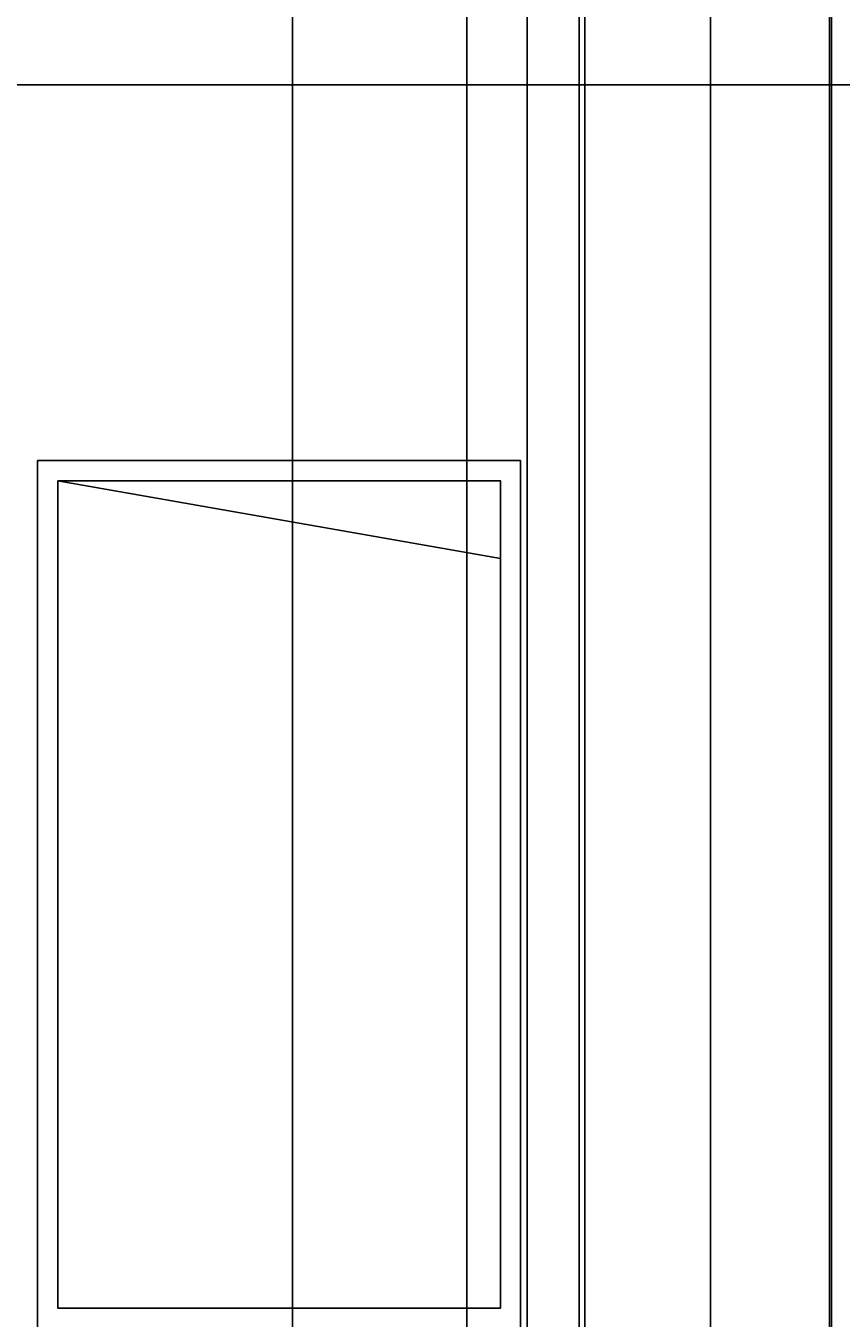
# Model space of a CAD drawing. Units: inches. Extents: x 69 to 650, y -16 to 573.
# Tile 5 of 26: x 264 to 345, y 89 to 218. Entities that reach past the tile are written whole.
import ezdxf

# ---------------------------------------------------------------- set-up
doc = ezdxf.new("R2010")
doc.units = ezdxf.units.IN
doc.header["$MEASUREMENT"] = 0
doc.layers.add('A-ANNO-DIMS', color=2, linetype='Continuous', lineweight=18)
doc.layers.add('A-DOOR', color=3, linetype='Continuous', lineweight=25)
doc.styles.get("Standard").update_dxf_attribs({"font": 'arial.ttf'})
doc.dimstyles.get("Standard").update_dxf_attribs({"dimtxt": 0.8125, "dimasz": 0.18, "dimexe": 0.18, "dimexo": 0.0625, "dimgap": 0.09, "dimtad": 0, "dimtih": 1, "dimtoh": 1, "dimdec": 4, "dimzin": 0, "dimdsep": 46, "dimlunit": 4, "dimtxsty": 'Standard', "dimcen": 0.09, "dimadec": 0, "dimazin": 0, "dimtfac": 1, "dimtdec": 4, "dimtofl": 0, "dimtmove": 0, "dimatfit": 3, "dimfxl": 1, "dimtolj": 1, "dimtzin": 0, "dimarcsym": 0})

# ---------------------------------------------------------------- blocks, each defined once
blk = doc.blocks.new('*D19')
at = {"layer": 'A-ANNO-DIMS', "color": 0, "lineweight": -2, "transparency": 16777216}
for p, q in [((99.56, 471.72), (99.56, 572.74)), ((99.74, 572.56), (358.57, 572.56)), ((619.38, 572.56), (360.54, 572.56)), ((619.56, 87.99), (619.56, 572.74))]:
    blk.add_line(p, q, dxfattribs=at)
at = {"layer": 'A-ANNO-DIMS', "color": 0, "transparency": 16777216}
for points in [[(99.74, 572.59), (99.74, 572.53), (99.56, 572.56)], [(619.38, 572.59), (619.38, 572.53), (619.56, 572.56)]]:
    blk.add_solid(points, dxfattribs=at)
at = {"layer": 'Defpoints', "color": 0, "transparency": 16777216}
for p in [(619.56, 572.56), (99.56, 471.66), (619.56, 87.93)]:
    blk.add_point(p, dxfattribs=at)
at = {"layer": 'A-ANNO-DIMS', "color": 0, "transparency": 16777216, "insert": (359.56, 572.56), "char_height": 0.812, "attachment_point": 5}
blk.add_mtext('\\A1;520', dxfattribs=at)
blk = doc.blocks.new('*D24')
at = {"layer": 'A-ANNO-DIMS', "color": 0, "lineweight": -2, "transparency": 16777216}
for p, q in [((441.88, 211.65), (70.98, 211.65)), ((71.16, 211.47), (71.16, 207.04)), ((71.16, 201.6), (71.16, 206.03)), ((173.51, 201.42), (70.98, 201.42))]:
    blk.add_line(p, q, dxfattribs=at)
at = {"layer": 'A-ANNO-DIMS', "color": 0, "transparency": 16777216}
for points in [[(71.13, 211.47), (71.19, 211.47), (71.16, 211.65)], [(71.13, 201.6), (71.19, 201.6), (71.16, 201.42)]]:
    blk.add_solid(points, dxfattribs=at)
at = {"layer": 'Defpoints', "color": 0, "transparency": 16777216}
for p in [(71.16, 211.65), (441.94, 211.65), (173.58, 201.42)]:
    blk.add_point(p, dxfattribs=at)
at = {"layer": 'A-ANNO-DIMS', "color": 0, "transparency": 16777216, "insert": (71.16, 206.54), "char_height": 0.812, "attachment_point": 5}
blk.add_mtext('\\A1;10.229', dxfattribs=at)
blk = doc.blocks.new('*D25')
at = {"layer": 'A-ANNO-DIMS', "color": 0, "lineweight": -2, "transparency": 16777216}
for p, q in [((99.49, 243.93), (70.98, 243.93)), ((71.16, 243.75), (71.16, 228.3)), ((71.16, 211.83), (71.16, 227.29)), ((441.88, 211.65), (70.98, 211.65))]:
    blk.add_line(p, q, dxfattribs=at)
at = {"layer": 'A-ANNO-DIMS', "color": 0, "transparency": 16777216}
for points in [[(71.13, 243.75), (71.19, 243.75), (71.16, 243.93)], [(71.13, 211.83), (71.19, 211.83), (71.16, 211.65)]]:
    blk.add_solid(points, dxfattribs=at)
at = {"layer": 'Defpoints', "color": 0, "transparency": 16777216}
for p in [(71.16, 243.93), (99.56, 243.93), (441.94, 211.65)]:
    blk.add_point(p, dxfattribs=at)
at = {"layer": 'A-ANNO-DIMS', "color": 0, "transparency": 16777216, "insert": (71.16, 227.79), "char_height": 0.812, "attachment_point": 5}
blk.add_mtext('\\A1;32.28', dxfattribs=at)
blk = doc.blocks.new('*D30')
at = {"layer": 'A-ANNO-DIMS', "color": 0, "lineweight": -2, "transparency": 16777216}
for p, q in [((352.94, 174.2), (352.94, 35.35)), ((313.14, 87.92), (313.14, 35.35)), ((313.32, 35.53), (331.9, 35.53)), ((352.76, 35.53), (334.19, 35.53))]:
    blk.add_line(p, q, dxfattribs=at)
at = {"layer": 'A-ANNO-DIMS', "color": 0, "transparency": 16777216}
for points in [[(313.32, 35.56), (313.32, 35.5), (313.14, 35.53)], [(352.76, 35.56), (352.76, 35.5), (352.94, 35.53)]]:
    blk.add_solid(points, dxfattribs=at)
at = {"layer": 'Defpoints', "color": 0, "transparency": 16777216}
for p in [(352.94, 174.27), (313.14, 87.99), (352.94, 35.53)]:
    blk.add_point(p, dxfattribs=at)
at = {"layer": 'A-ANNO-DIMS', "color": 0, "transparency": 16777216, "insert": (333.04, 35.53), "char_height": 0.812, "attachment_point": 5}
blk.add_mtext('\\A1;39.8', dxfattribs=at)
blk = doc.blocks.new('*D37')
at = {"layer": 'A-ANNO-DIMS', "color": 0, "lineweight": -2, "transparency": 16777216}
for p, q in [((307.8, 384.84), (307.8, 35.35)), ((290.45, 372.93), (290.45, 35.35)), ((290.63, 35.53), (297.7, 35.53)), ((307.62, 35.53), (300.55, 35.53))]:
    blk.add_line(p, q, dxfattribs=at)
at = {"layer": 'A-ANNO-DIMS', "color": 0, "transparency": 16777216}
for points in [[(290.63, 35.56), (290.63, 35.5), (290.45, 35.53)], [(307.62, 35.56), (307.62, 35.5), (307.8, 35.53)]]:
    blk.add_solid(points, dxfattribs=at)
at = {"layer": 'Defpoints', "color": 0, "transparency": 16777216}
for p in [(307.8, 384.9), (290.45, 372.99), (307.8, 35.53)]:
    blk.add_point(p, dxfattribs=at)
at = {"layer": 'A-ANNO-DIMS', "color": 0, "transparency": 16777216, "insert": (299.12, 35.53), "char_height": 0.812, "attachment_point": 5}
blk.add_mtext('\\A1;17.35', dxfattribs=at)
blk = doc.blocks.new('*D38')
at = {"layer": 'A-ANNO-DIMS', "color": 0, "lineweight": -2, "transparency": 16777216}
for p, q in [((307.8, 384.84), (307.8, 35.35)), ((390.43, 384.84), (390.43, 35.35)), ((307.98, 35.53), (347.65, 35.53)), ((390.25, 35.53), (350.57, 35.53))]:
    blk.add_line(p, q, dxfattribs=at)
at = {"layer": 'A-ANNO-DIMS', "color": 0, "transparency": 16777216}
for points in [[(307.98, 35.56), (307.98, 35.5), (307.8, 35.53)], [(390.25, 35.56), (390.25, 35.5), (390.43, 35.53)]]:
    blk.add_solid(points, dxfattribs=at)
at = {"layer": 'Defpoints', "color": 0, "transparency": 16777216}
for p in [(307.8, 384.9), (390.43, 384.9), (390.43, 35.53)]:
    blk.add_point(p, dxfattribs=at)
at = {"layer": 'A-ANNO-DIMS', "color": 0, "transparency": 16777216, "insert": (349.11, 35.53), "char_height": 0.812, "attachment_point": 5}
blk.add_mtext('\\A1;82.63', dxfattribs=at)
blk = doc.blocks.new('*D64')
at = {"layer": 'A-ANNO-DIMS', "color": 0, "lineweight": -2, "transparency": 16777216}
for p, q in [((319.55, 393.8), (319.55, 35.35)), ((344.08, 393.8), (344.08, 35.35)), ((319.73, 35.53), (330.35, 35.53)), ((343.9, 35.53), (333.28, 35.53))]:
    blk.add_line(p, q, dxfattribs=at)
at = {"layer": 'A-ANNO-DIMS', "color": 0, "transparency": 16777216}
for points in [[(319.73, 35.56), (319.73, 35.5), (319.55, 35.53)], [(343.9, 35.56), (343.9, 35.5), (344.08, 35.53)]]:
    blk.add_solid(points, dxfattribs=at)
at = {"layer": 'Defpoints', "color": 0, "transparency": 16777216}
for p in [(319.55, 393.86), (344.08, 393.86), (344.08, 35.53)]:
    blk.add_point(p, dxfattribs=at)
at = {"layer": 'A-ANNO-DIMS', "color": 0, "transparency": 16777216, "insert": (331.82, 35.53), "char_height": 0.812, "attachment_point": 5}
blk.add_mtext('\\A1;24.53', dxfattribs=at)
blk = doc.blocks.new('*D65')
at = {"layer": 'A-ANNO-DIMS', "color": 0, "lineweight": -2, "transparency": 16777216}
for p, q in [((344.08, 393.8), (344.08, 35.35)), ((368.88, 393.8), (368.88, 35.35)), ((344.26, 35.53), (355.33, 35.53)), ((368.7, 35.53), (357.63, 35.53))]:
    blk.add_line(p, q, dxfattribs=at)
at = {"layer": 'A-ANNO-DIMS', "color": 0, "transparency": 16777216}
for points in [[(344.26, 35.56), (344.26, 35.5), (344.08, 35.53)], [(368.7, 35.56), (368.7, 35.5), (368.88, 35.53)]]:
    blk.add_solid(points, dxfattribs=at)
at = {"layer": 'Defpoints', "color": 0, "transparency": 16777216}
for p in [(344.08, 393.86), (368.88, 393.86), (368.88, 35.53)]:
    blk.add_point(p, dxfattribs=at)
at = {"layer": 'A-ANNO-DIMS', "color": 0, "transparency": 16777216, "insert": (356.48, 35.53), "char_height": 0.812, "attachment_point": 5}
blk.add_mtext('\\A1;24.8', dxfattribs=at)
blk = doc.blocks.new('*D66')
at = {"layer": 'A-ANNO-DIMS', "color": 0, "lineweight": -2, "transparency": 16777216}
for p, q in [((313.81, 263.46), (313.81, 35.35)), ((318.98, 263.46), (318.98, 35.35)), ((313.99, 35.53), (314.93, 35.53)), ((318.8, 35.53), (317.85, 35.53))]:
    blk.add_line(p, q, dxfattribs=at)
at = {"layer": 'A-ANNO-DIMS', "color": 0, "transparency": 16777216}
for points in [[(313.99, 35.56), (313.99, 35.5), (313.81, 35.53)], [(318.8, 35.56), (318.8, 35.5), (318.98, 35.53)]]:
    blk.add_solid(points, dxfattribs=at)
at = {"layer": 'Defpoints', "color": 0, "transparency": 16777216}
for p in [(313.81, 263.53), (318.98, 263.53), (318.98, 35.53)]:
    blk.add_point(p, dxfattribs=at)
at = {"layer": 'A-ANNO-DIMS', "color": 0, "transparency": 16777216, "insert": (316.39, 35.53), "char_height": 0.812, "attachment_point": 5}
blk.add_mtext('\\A1;5.174', dxfattribs=at)
blk = doc.blocks.new('*D67')
at = {"layer": 'A-ANNO-DIMS', "color": 0, "lineweight": -2, "transparency": 16777216}
for p, q in [((318.98, 263.46), (318.98, 35.35)), ((332.05, 263.46), (332.05, 35.35)), ((319.16, 35.53), (324.09, 35.53)), ((331.87, 35.53), (326.94, 35.53))]:
    blk.add_line(p, q, dxfattribs=at)
at = {"layer": 'A-ANNO-DIMS', "color": 0, "transparency": 16777216}
for points in [[(319.16, 35.56), (319.16, 35.5), (318.98, 35.53)], [(331.87, 35.56), (331.87, 35.5), (332.05, 35.53)]]:
    blk.add_solid(points, dxfattribs=at)
at = {"layer": 'Defpoints', "color": 0, "transparency": 16777216}
for p in [(318.98, 263.53), (332.05, 263.53), (332.05, 35.53)]:
    blk.add_point(p, dxfattribs=at)
at = {"layer": 'A-ANNO-DIMS', "color": 0, "transparency": 16777216, "insert": (325.52, 35.53), "char_height": 0.812, "attachment_point": 5}
blk.add_mtext('\\A1;13.07', dxfattribs=at)
blk = doc.blocks.new('*D68')
at = {"layer": 'A-ANNO-DIMS', "color": 0, "lineweight": -2, "transparency": 16777216}
for p, q in [((332.05, 263.46), (332.05, 35.35)), ((343.89, 263.46), (343.89, 35.35)), ((332.23, 35.53), (336.23, 35.53)), ((343.71, 35.53), (339.71, 35.53))]:
    blk.add_line(p, q, dxfattribs=at)
at = {"layer": 'A-ANNO-DIMS', "color": 0, "transparency": 16777216}
for points in [[(332.23, 35.56), (332.23, 35.5), (332.05, 35.53)], [(343.71, 35.56), (343.71, 35.5), (343.89, 35.53)]]:
    blk.add_solid(points, dxfattribs=at)
at = {"layer": 'Defpoints', "color": 0, "transparency": 16777216}
for p in [(332.05, 263.53), (343.89, 263.53), (343.89, 35.53)]:
    blk.add_point(p, dxfattribs=at)
at = {"layer": 'A-ANNO-DIMS', "color": 0, "transparency": 16777216, "insert": (337.97, 35.53), "char_height": 0.812, "attachment_point": 5}
blk.add_mtext('\\A1;11.839', dxfattribs=at)
blk = doc.blocks.new('*D69')
at = {"layer": 'A-ANNO-DIMS', "color": 0, "lineweight": -2, "transparency": 16777216}
for p, q in [((343.89, 263.46), (343.89, 35.35)), ((357.51, 263.46), (357.51, 35.35)), ((344.07, 35.53), (349.28, 35.53)), ((357.33, 35.53), (352.12, 35.53))]:
    blk.add_line(p, q, dxfattribs=at)
at = {"layer": 'A-ANNO-DIMS', "color": 0, "transparency": 16777216}
for points in [[(344.07, 35.56), (344.07, 35.5), (343.89, 35.53)], [(357.33, 35.56), (357.33, 35.5), (357.51, 35.53)]]:
    blk.add_solid(points, dxfattribs=at)
at = {"layer": 'Defpoints', "color": 0, "transparency": 16777216}
for p in [(343.89, 263.53), (357.51, 263.53), (357.51, 35.53)]:
    blk.add_point(p, dxfattribs=at)
at = {"layer": 'A-ANNO-DIMS', "color": 0, "transparency": 16777216, "insert": (350.7, 35.53), "char_height": 0.812, "attachment_point": 5}
blk.add_mtext('\\A1;13.62', dxfattribs=at)

msp = doc.modelspace()

# ---------------------------------------------------------------- linework, layer by layer
at = {"layer": 'A-DOOR'}
msp.add_line((267.0952, 172.2666), (311.1416, 164.5445), dxfattribs=at)
for points in [[(265.0952, 174.2666), (313.1416, 174.2666), (313.1416, 87.985), (265.0952, 87.985)], [(267.0952, 172.2666), (311.1416, 172.2666), (311.1416, 89.985), (267.0952, 89.985)]]:
    msp.add_lwpolyline(points, close=True, dxfattribs=at)

# ---------------------------------------------------------------- dimensions: what is measured, and where the dimension line sits
at = {"layer": 'A-ANNO-DIMS'}
for base, p1, p2, override, picture, middle in [((619.555, 572.5573), (99.556, 471.6595), (619.555, 87.93), {"dimdec": 0, "dimlfac": 1, "dimrnd": 0, "dimzin": 0, "dimdsep": 46, "dimlunit": 2}, '*D19', (359.5555, 572.5573)), ((344.0804, 35.53), (319.5513, 393.8576), (344.0804, 393.8576), {"dimdec": 2, "dimlfac": 1, "dimrnd": 0, "dimzin": 0, "dimdsep": 46, "dimlunit": 2}, '*D64', (331.8159, 35.53)), ((368.881, 35.53), (344.0804, 393.8576), (368.881, 393.8576), {"dimdec": 1, "dimlfac": 1, "dimrnd": 0, "dimzin": 0, "dimdsep": 46, "dimlunit": 2}, '*D65', (356.4807, 35.53)), ((307.7955, 35.53), (290.4461, 372.9907), (307.7955, 384.8986), {"dimdec": 2, "dimlfac": 1, "dimrnd": 0, "dimzin": 0, "dimdsep": 46, "dimlunit": 2}, '*D37', (299.1208, 35.53)), ((390.4291, 35.53), (307.7955, 384.8986), (390.4291, 384.8986), {"dimdec": 2, "dimlfac": 1, "dimrnd": 0, "dimzin": 0, "dimdsep": 46, "dimlunit": 2}, '*D38', (349.1123, 35.53)), ((318.9804, 35.53), (313.8067, 263.5253), (318.9804, 263.5253), {"dimdec": 3, "dimlfac": 1, "dimrnd": 0, "dimzin": 0, "dimdsep": 46, "dimlunit": 2}, '*D66', (316.3936, 35.53)), ((332.0516, 35.53), (318.9804, 263.5253), (332.0516, 263.5253), {"dimdec": 2, "dimlfac": 1, "dimrnd": 0, "dimzin": 0, "dimdsep": 46, "dimlunit": 2}, '*D67', (325.516, 35.53)), ((343.8902, 35.53), (332.0516, 263.5253), (343.8902, 263.5253), {"dimdec": 3, "dimlfac": 1, "dimrnd": 0, "dimzin": 0, "dimdsep": 46, "dimlunit": 2}, '*D68', (337.9709, 35.53)), ((357.5106, 35.53), (343.8902, 263.5253), (357.5106, 263.5253), {"dimdec": 2, "dimlfac": 1, "dimrnd": 0, "dimzin": 0, "dimdsep": 46, "dimlunit": 2}, '*D69', (350.7004, 35.53)), ((352.9415, 35.53), (313.1416, 87.985), (352.9415, 174.2666), {"dimdec": 1, "dimlfac": 1, "dimrnd": 0, "dimzin": 0, "dimdsep": 46, "dimlunit": 2}, '*D30', (333.0415, 35.53))]:
    dim = msp.add_linear_dim(base=base, p1=p1, p2=p2, dimstyle='Standard', override=override, dxfattribs=at)
    dim.commit()
    dim.dimension.update_dxf_attribs({"geometry": picture, "text_midpoint": middle})
for base, p1, p2, override, picture, middle in [((71.156, 243.93), (441.9398, 211.6519), (99.556, 243.93), {"dimdec": 2, "dimlfac": 1, "dimrnd": 0, "dimzin": 0, "dimdsep": 46, "dimlunit": 2}, '*D25', (71.156, 227.7909)), ((71.156, 211.6519), (173.5769, 201.4229), (441.9398, 211.6519), {"dimdec": 3, "dimlfac": 1, "dimrnd": 0, "dimzin": 0, "dimdsep": 46, "dimlunit": 2}, '*D24', (71.156, 206.5374))]:
    dim = msp.add_linear_dim(base=base, p1=p1, p2=p2, angle=90, dimstyle='Standard', override=override, dxfattribs=at)
    dim.commit()
    dim.dimension.update_dxf_attribs({"geometry": picture, "text_midpoint": middle})

doc.saveas('drawing.dxf')
